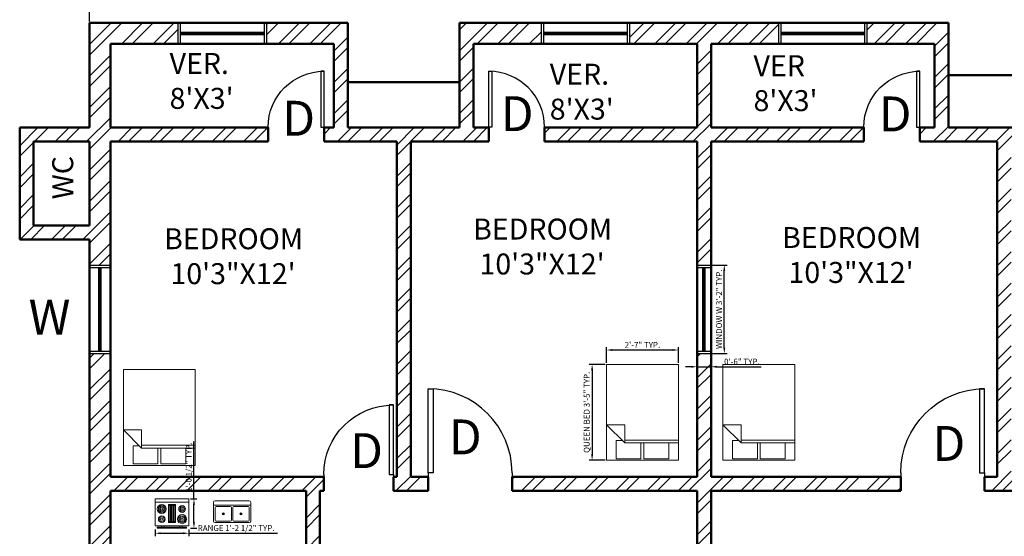
# Model space of a CAD drawing. Units: inches. Extents: x -31485 to -28799, y 18003 to 19130.
# Tile 13 of 15: x -29694 to -29271, y 18604 to 18825. Entities that reach past the tile are written whole.
import ezdxf

# ---------------------------------------------------------------- set-up
doc = ezdxf.new("R2010")
doc.units = ezdxf.units.IN
for name, color, linetype, lineweight in [('A-ANNO-DIMS', 2, 'Continuous', 18), ('A-ANNO-TEXT', 7, 'Continuous', 18), ('A-AREA-IDEN', 7, 'Continuous', 18), ('A-DOOR', 3, 'Continuous', 25), ('A-FLOR-FIXT', 9, 'Continuous', 18), ('A-FURN', 8, 'Continuous', 18), ('A-GLAZ', 4, 'Continuous', 25), ('A-WALL', 7, 'Continuous', 50), ('A-WALL-PATT', 8, 'Continuous', 13)]:
    doc.layers.add(name, color=color, linetype=linetype, lineweight=lineweight)
doc.styles.get("Standard").update_dxf_attribs({"font": 'arial.ttf'})
doc.dimstyles.new('ISO-25', dxfattribs={"dimtxt": 2.5, "dimasz": 2.5, "dimexe": 1.25, "dimexo": 0.625, "dimtad": 1, "dimdec": 0, "dimlunit": 3, "dimtxsty": 'Standard', "dimcen": 2.5, "dimadec": 0, "dimazin": 0, "dimtfac": 1, "dimtdec": 0, "dimtmove": 0, "dimatfit": 3, "dimfxl": 1, "dimarcsym": 0})

# ---------------------------------------------------------------- blocks, each defined once
blk = doc.blocks.new('*U8')
for p, q in [((0, 0), (0, -100)), ((750, 0), (750, -100))]:
    blk.add_line(p, q)
blk.add_lwpolyline([(0, 0), (0, 750), (43.75, 750), (43.75, 0)], close=True)
blk.add_arc((0, 0), 750, 0, 90)
blk = doc.blocks.new('Bed - Queen')
for p, q in [((0, -80.00003), (0, 0)), ((0, 0), (59.99999, 0)), ((59.99999, 0), (59.99999, -80.00003)), ((7.99999, -1.2), (28.79998, -1.2)), ((7.99999, -14.4), (7.99999, -1.2)), ((28.79998, -1.2), (28.79998, -14.4)), ((31.19999, -1.2), (51.99999, -1.2)), ((31.19999, -14.4), (31.19999, -1.2)), ((51.99999, -1.2), (51.99999, -16.4)), ((0, -14.4), (44.8, -14.4)), ((59.99999, -29.6), (44.8, -14.4)), ((44.8, -14.4), (44.8, -29.6)), ((51.99999, -16.4), (46.79936, -16.4)), ((44.8, -16.8), (0, -16.8)), ((44.8, -29.6), (59.99999, -29.6)), ((59.99999, -80.00003), (0, -80.00003))]:
    blk.add_line(p, q)
blk = doc.blocks.new('Range-Oven - 30 in top')
for p, q in [((0, -3), (30, -3)), ((12, -6), (18, -6)), ((13, -20), (13, -6)), ((14, -6), (14, -20)), ((15, -20), (15, -6)), ((16, -6), (16, -20)), ((17, -20), (17, -6)), ((6, -24), (6, -25)), ((8, -25), (8, -24)), ((18, -20), (12, -20)), ((22, -25), (22, -24)), ((24, -24), (24, -25))]:
    blk.add_line(p, q)
for points in [[(0, -24), (0, 0), (30, 0), (30, -24)], [(12, -21), (12, -5), (18, -5), (18, -21)], [(2, -26), (2, -25), (28, -25), (28, -26)]]:
    blk.add_lwpolyline(points, close=True)
for centre, radius in [((6, -9), 4), ((6, -9), 3), ((6, -9), 2), ((6, -9), 1), ((24, -9), 3), ((24, -9), 2), ((24, -9), 1), ((6, -18), 3), ((6, -18), 2), ((6, -18), 1), ((24, -18), 4), ((24, -18), 3), ((24, -18), 2), ((24, -18), 1)]:
    blk.add_circle(centre, radius)
blk = doc.blocks.new('Sink-double - 36 in top')
for p, q in [((-18, -4), (18, -4)), ((-0.75, -18.5), (-0.75, -6.5)), ((0.75, -6.5), (0.75, -18.5))]:
    blk.add_line(p, q)
for points in [[(-16.5, 0), (16.5, 0)], [(-18, -19.5), (-18, -1.5)], [(-16.5, -18.5), (-16.5, -6.5)], [(-15.5, -5.5), (-1.75, -5.5)], [(1.75, -5.5), (15.5, -5.5)], [(16.5, -6.5), (16.5, -18.5)], [(18, -1.5), (18, -19.5)], [(16.5, -21), (-16.5, -21)], [(-1.75, -19.5), (-15.5, -19.5)], [(15.5, -19.5), (1.75, -19.5)]]:
    blk.add_lwpolyline(points)
for centre, radius in [((-8.5, -12.5), 1), ((-8.5, -12.5), 0.5), ((8.5, -12.5), 1), ((8.5, -12.5), 0.5)]:
    blk.add_circle(centre, radius)
for centre, radius, start, end in [((-16.5, -1.5), 1.5, 90, 180), ((16.5, -1.5), 1.5, 0, 90), ((-15.5, -6.5), 1, 90, 180), ((-1.75, -6.5), 1, 0, 90), ((1.75, -6.5), 1, 90, 180), ((15.5, -6.5), 1, 0, 90), ((-15.5, -18.5), 1, 180, 270), ((-1.75, -18.5), 1, 270, 0), ((1.75, -18.5), 1, 180, 270), ((15.5, -18.5), 1, 270, 0), ((-16.5, -19.5), 1.5, 180, 270), ((16.5, -19.5), 1.5, 270, 0)]:
    blk.add_arc(centre, radius, start, end)
blk = doc.blocks.new('*D204')
at = {"layer": 'A-ANNO-DIMS', "color": 0, "lineweight": -2, "transparency": 16777216}
for p, q in [((-29663.82, 18824.74), (-29663.82, 18894.35)), ((-29661.32, 18893.1), (-29118.32, 18893.1)), ((-29115.82, 18824.74), (-29115.82, 18894.35))]:
    blk.add_line(p, q, dxfattribs=at)
at = {"layer": 'A-ANNO-DIMS', "color": 0, "transparency": 16777216}
for points in [[(-29661.32, 18893.52), (-29661.32, 18892.68), (-29663.82, 18893.1)], [(-29118.32, 18893.52), (-29118.32, 18892.68), (-29115.82, 18893.1)]]:
    blk.add_solid(points, dxfattribs=at)
at = {"layer": 'Defpoints', "color": 0, "transparency": 16777216}
for p in [(-29115.82, 18893.1), (-29663.82, 18824.12), (-29115.82, 18824.12)]:
    blk.add_point(p, dxfattribs=at)
at = {"layer": 'A-ANNO-DIMS', "color": 0, "transparency": 16777216, "insert": (-29389.82, 18901.9), "char_height": 2.5, "attachment_point": 5}
blk.add_mtext('{\\H6.4x;45\'-8"}', dxfattribs=at)
blk = doc.blocks.new('WIN-900-W9')
for p, q in [((-29982.21, 18824.12), (-29982.21, 18815.12)), ((-29981.21, 18824.12), (-29981.21, 18815.12)), ((-29945.21, 18824.12), (-29945.21, 18815.12)), ((-29944.21, 18824.12), (-29944.21, 18815.12)), ((-29981.21, 18820.12), (-29945.21, 18820.12)), ((-29981.21, 18819.62), (-29945.21, 18819.62)), ((-29981.21, 18819.12), (-29945.21, 18819.12))]:
    blk.add_line(p, q)
blk = doc.blocks.new('WIN-900-W6')
for p, q in [((-30183.21, 18720.12), (-30177.21, 18720.12)), ((-30183.21, 18719.12), (-30177.21, 18719.12)), ((-30180.71, 18683.12), (-30180.71, 18719.12)), ((-30180.21, 18683.12), (-30180.21, 18719.12)), ((-30179.71, 18683.12), (-30179.71, 18719.12)), ((-30183.21, 18683.12), (-30177.21, 18683.12)), ((-30183.21, 18682.12), (-30177.21, 18682.12))]:
    blk.add_line(p, q)
blk = doc.blocks.new('*D212')
at = {"layer": 'A-ANNO-DIMS', "color": 0, "lineweight": -2, "transparency": 16777216}
for p, q in [((-29396.2, 18720.12), (-29389.87, 18720.12)), ((-29391.12, 18684.62), (-29391.12, 18717.62)), ((-29396.2, 18682.12), (-29389.87, 18682.12))]:
    blk.add_line(p, q, dxfattribs=at)
at = {"layer": 'A-ANNO-DIMS', "color": 0, "transparency": 16777216}
for points in [[(-29391.54, 18717.62), (-29390.7, 18717.62), (-29391.12, 18720.12)], [(-29391.54, 18684.62), (-29390.7, 18684.62), (-29391.12, 18682.12)]]:
    blk.add_solid(points, dxfattribs=at)
at = {"layer": 'Defpoints', "color": 0, "transparency": 16777216}
for p in [(-29396.82, 18720.12), (-29391.12, 18720.12), (-29396.82, 18682.12)]:
    blk.add_point(p, dxfattribs=at)
at = {"layer": 'A-ANNO-DIMS', "color": 0, "transparency": 16777216, "insert": (-29393.04, 18701.12), "char_height": 2.5, "attachment_point": 5, "rotation": 90}
blk.add_mtext('WINDOW W 3\'-2" TYP.', dxfattribs=at)
blk = doc.blocks.new('*D213')
at = {"layer": 'A-ANNO-DIMS', "color": 0, "lineweight": -2, "transparency": 16777216}
for p, q in [((-29402.82, 18681.49), (-29402.82, 18675.17)), ((-29396.82, 18681.49), (-29396.82, 18675.17)), ((-29405.32, 18676.42), (-29407.82, 18676.42)), ((-29402.82, 18676.42), (-29396.82, 18676.42)), ((-29394.32, 18676.42), (-29375.33, 18676.42))]:
    blk.add_line(p, q, dxfattribs=at)
at = {"layer": 'A-ANNO-DIMS', "color": 0, "transparency": 16777216}
for points in [[(-29405.32, 18676.83), (-29405.32, 18676), (-29402.82, 18676.42)], [(-29394.32, 18676.83), (-29394.32, 18676), (-29396.82, 18676.42)]]:
    blk.add_solid(points, dxfattribs=at)
at = {"layer": 'Defpoints', "color": 0, "transparency": 16777216}
for p in [(-29402.82, 18682.12), (-29396.82, 18682.12), (-29396.82, 18676.42)]:
    blk.add_point(p, dxfattribs=at)
at = {"layer": 'A-ANNO-DIMS', "color": 0, "transparency": 16777216, "insert": (-29383.58, 18678.32), "char_height": 2.5, "attachment_point": 5}
blk.add_mtext('0\'-6" TYP.', dxfattribs=at)
blk = doc.blocks.new('*D222')
at = {"layer": 'A-ANNO-DIMS', "color": 0, "lineweight": -2, "transparency": 16777216}
for p, q in [((-29442.35, 18677.44), (-29449.15, 18677.44)), ((-29447.9, 18674.94), (-29447.9, 18638.78)), ((-29442.35, 18636.28), (-29449.15, 18636.28))]:
    blk.add_line(p, q, dxfattribs=at)
at = {"layer": 'A-ANNO-DIMS', "color": 0, "transparency": 16777216}
for points in [[(-29448.32, 18674.94), (-29447.48, 18674.94), (-29447.9, 18677.44)], [(-29448.32, 18638.78), (-29447.48, 18638.78), (-29447.9, 18636.28)]]:
    blk.add_solid(points, dxfattribs=at)
at = {"layer": 'Defpoints', "color": 0, "transparency": 16777216}
for p in [(-29441.73, 18677.44), (-29447.9, 18636.28), (-29441.73, 18636.28)]:
    blk.add_point(p, dxfattribs=at)
at = {"layer": 'A-ANNO-DIMS', "color": 0, "transparency": 16777216, "insert": (-29449.9, 18656.86), "char_height": 2.5, "attachment_point": 5, "rotation": 90}
blk.add_mtext('QUEEN BED 3\'-5" TYP.', dxfattribs=at)
blk = doc.blocks.new('*D223')
at = {"layer": 'A-ANNO-DIMS', "color": 0, "lineweight": -2, "transparency": 16777216}
for p, q in [((-29441.73, 18678.06), (-29441.73, 18684.86)), ((-29410.86, 18678.06), (-29410.86, 18684.86)), ((-29413.36, 18683.61), (-29439.23, 18683.61))]:
    blk.add_line(p, q, dxfattribs=at)
at = {"layer": 'A-ANNO-DIMS', "color": 0, "transparency": 16777216}
for points in [[(-29439.23, 18684.03), (-29439.23, 18683.19), (-29441.73, 18683.61)], [(-29413.36, 18684.03), (-29413.36, 18683.19), (-29410.86, 18683.61)]]:
    blk.add_solid(points, dxfattribs=at)
at = {"layer": 'Defpoints', "color": 0, "transparency": 16777216}
for p in [(-29441.73, 18683.61), (-29441.73, 18677.44), (-29410.86, 18677.44)]:
    blk.add_point(p, dxfattribs=at)
at = {"layer": 'A-ANNO-DIMS', "color": 0, "transparency": 16777216, "insert": (-29426.29, 18685.49), "char_height": 2.5, "attachment_point": 5}
blk.add_mtext('2\'-7" TYP.', dxfattribs=at)
blk = doc.blocks.new('*D250')
at = {"layer": 'A-ANNO-DIMS', "color": 0, "lineweight": -2, "transparency": 16777216}
for p, q in [((-29635.69, 18606.46), (-29635.69, 18603.66)), ((-29633.19, 18604.91), (-29623.64, 18604.91)), ((-29621.14, 18606.46), (-29621.14, 18603.66)), ((-29621.14, 18604.91), (-29583.06, 18604.91))]:
    blk.add_line(p, q, dxfattribs=at)
at = {"layer": 'A-ANNO-DIMS', "color": 0, "transparency": 16777216}
for points in [[(-29633.19, 18605.32), (-29633.19, 18604.49), (-29635.69, 18604.91)], [(-29623.64, 18605.32), (-29623.64, 18604.49), (-29621.14, 18604.91)]]:
    blk.add_solid(points, dxfattribs=at)
at = {"layer": 'Defpoints', "color": 0, "transparency": 16777216}
for p in [(-29635.69, 18607.09), (-29621.14, 18607.09), (-29621.14, 18604.91)]:
    blk.add_point(p, dxfattribs=at)
at = {"layer": 'A-ANNO-DIMS', "color": 0, "transparency": 16777216, "insert": (-29600.85, 18606.82), "char_height": 2.5, "attachment_point": 5}
blk.add_mtext('RANGE 1\'-2 1/2" TYP.', dxfattribs=at)
blk = doc.blocks.new('*D251')
at = {"layer": 'A-ANNO-DIMS', "color": 0, "lineweight": -2, "transparency": 16777216}
for p, q in [((-29618.95, 18619.7), (-29618.95, 18644.28)), ((-29620.51, 18619.7), (-29617.7, 18619.7)), ((-29618.95, 18609.59), (-29618.95, 18617.2)), ((-29620.51, 18607.09), (-29617.7, 18607.09))]:
    blk.add_line(p, q, dxfattribs=at)
at = {"layer": 'A-ANNO-DIMS', "color": 0, "transparency": 16777216}
for points in [[(-29619.37, 18617.2), (-29618.54, 18617.2), (-29618.95, 18619.7)], [(-29619.37, 18609.59), (-29618.54, 18609.59), (-29618.95, 18607.09)]]:
    blk.add_solid(points, dxfattribs=at)
at = {"layer": 'Defpoints', "color": 0, "transparency": 16777216}
for p in [(-29621.14, 18619.7), (-29618.95, 18619.7), (-29621.14, 18607.09)]:
    blk.add_point(p, dxfattribs=at)
at = {"layer": 'A-ANNO-DIMS', "color": 0, "transparency": 16777216, "insert": (-29620.87, 18633.24), "char_height": 2.5, "attachment_point": 5, "rotation": 90}
blk.add_mtext('1\'-0 1/2" TYP.', dxfattribs=at)

msp = doc.modelspace()

# ---------------------------------------------------------------- hatches: boundary and pattern name
at = {"layer": 'A-WALL-PATT'}
h = msp.add_hatch(dxfattribs=at)
h.set_pattern_fill('ANSI32', color=256)
h.set_pattern_definition([(45, (-227.67, 0), (-6.735192, 6.735192), []), (45, (-223.18, 0), (-6.735192, 6.735192), [])])
h.paths.add_polyline_path([(-29507.82, 18213.12), (-29493.82, 18213.12), (-29493.82, 18219.12), (-29507.82, 18219.12), (-29507.82, 18309.12), (-29504.3, 18309.12), (-29504.3, 18315.12), (-29513.82, 18315.12), (-29513.82, 18243.12), (-29654.82, 18243.12), (-29654.82, 18265.36), (-29663.82, 18265.36), (-29663.82, 18180.12), (-29603.32, 18180.12), (-29603.32, 18189.12), (-29654.82, 18189.12), (-29654.82, 18237.12), (-29513.82, 18237.12), (-29513.82, 18189.12), (-29565.32, 18189.12), (-29565.32, 18180.12), (-29507.82, 18180.12)])
h.paths.add_polyline_path([(-29408.82, 18189.12), (-29447.82, 18189.12), (-29447.82, 18371.74), (-29453.82, 18371.74), (-29453.82, 18365.12), (-29476.66, 18365.12), (-29476.66, 18359.12), (-29453.82, 18359.12), (-29453.82, 18315.12), (-29480.3, 18315.12), (-29480.3, 18309.12), (-29453.82, 18309.12), (-29453.82, 18219.12), (-29467.82, 18219.12), (-29467.82, 18213.12), (-29453.82, 18213.12), (-29453.82, 18180.12), (-29408.82, 18180.12)])
h.paths.add_polyline_path([(-29325.82, 18213.12), (-29311.82, 18213.12), (-29311.82, 18219.12), (-29325.82, 18219.12), (-29325.82, 18309.12), (-29298.35, 18309.12), (-29298.35, 18315.12), (-29325.82, 18315.12), (-29325.82, 18359.12), (-29304.41, 18359.12), (-29304.41, 18365.12), (-29325.82, 18365.12), (-29325.82, 18371.25), (-29331.82, 18371.25), (-29331.82, 18189.12), (-29370.82, 18189.12), (-29370.82, 18180.12), (-29325.82, 18180.12)])
h.paths.add_polyline_path([(-29265.82, 18237.12), (-29124.82, 18237.12), (-29124.82, 18189.12), (-29176.32, 18189.12), (-29176.32, 18180.12), (-29115.82, 18180.12), (-29115.82, 18268.84), (-29124.82, 18268.84), (-29124.82, 18243.12), (-29265.82, 18243.12), (-29265.82, 18315.12), (-29274.35, 18315.12), (-29274.35, 18309.12), (-29271.82, 18309.12), (-29271.82, 18219.12), (-29285.82, 18219.12), (-29285.82, 18213.12), (-29271.82, 18213.12), (-29271.82, 18180.12), (-29214.32, 18180.12), (-29214.32, 18189.12), (-29265.82, 18189.12)])
h.paths.add_polyline_path([(-29209.82, 18365.12), (-29262.82, 18365.12), (-29268.41, 18365.12), (-29268.41, 18359.12), (-29209.82, 18359.12)])
h.paths.add_polyline_path([(-29085.82, 18365.12), (-29115.82, 18365.12), (-29115.82, 18400.12), (-29124.82, 18400.12), (-29124.82, 18365.12), (-29171.82, 18365.12), (-29171.82, 18359.12), (-29124.82, 18359.12), (-29124.82, 18306.84), (-29115.82, 18306.84), (-29115.82, 18317.12), (-29085.82, 18317.12)])
h.paths.add_polyline_path([(-29115.82, 18359.12), (-29091.82, 18359.12), (-29091.82, 18323.12), (-29115.82, 18323.12)], flags=16)
h.paths.add_polyline_path([(-29607.82, 18365.12), (-29654.82, 18365.12), (-29654.82, 18400.12), (-29663.82, 18400.12), (-29663.82, 18365.12), (-29693.82, 18365.12), (-29693.82, 18317.12), (-29663.82, 18317.12), (-29663.82, 18303.36), (-29654.82, 18303.36), (-29654.82, 18359.12), (-29607.82, 18359.12)])
h.paths.add_polyline_path([(-29663.82, 18359.12), (-29663.82, 18323.12), (-29687.82, 18323.12), (-29687.82, 18359.12)], flags=16)
h.paths.add_polyline_path([(-29512.66, 18365.12), (-29516.82, 18365.12), (-29569.82, 18365.12), (-29569.82, 18359.12), (-29512.66, 18359.12)])
h.paths.add_polyline_path([(-29654.82, 18473.12), (-29553.73, 18473.12), (-29553.73, 18479.12), (-29564.82, 18479.12), (-29564.82, 18500.25), (-29569.57, 18500.25, -0.011537), (-29570.67, 18500.25), (-29570.82, 18500.25), (-29570.82, 18479.12), (-29675.82, 18479.12), (-29675.82, 18493.12), (-29681.82, 18493.12), (-29681.82, 18473.12), (-29663.82, 18473.12), (-29663.82, 18438.12), (-29654.82, 18438.12)])
h.paths.add_polyline_path([(-29564.82, 18547.44), (-29570.82, 18547.44), (-29570.82, 18539.12), (-29654.82, 18539.12), (-29654.82, 18562.12), (-29663.82, 18562.12), (-29663.82, 18539.12), (-29681.82, 18539.12), (-29681.82, 18519.12), (-29675.82, 18519.12), (-29675.82, 18533.12), (-29570.82, 18533.12), (-29570.82, 18524.25), (-29564.82, 18524.25)])
h.paths.add_polyline_path([(-29563.19, 18629.12), (-29654.82, 18629.12), (-29654.82, 18682.12), (-29663.82, 18682.12), (-29663.82, 18600.12), (-29654.82, 18600.12), (-29654.82, 18623.12), (-29570.82, 18623.12), (-29570.82, 18583.44), (-29566.85, 18583.44), (-29564.82, 18583.44), (-29564.82, 18623.12), (-29563.19, 18623.12)])
h.paths.add_polyline_path([(-29315.33, 18629.12), (-29396.82, 18629.12), (-29396.82, 18682.12), (-29402.82, 18682.12), (-29402.82, 18629.12), (-29482.28, 18629.12), (-29482.28, 18626.12), (-29482.28, 18623.12), (-29402.82, 18623.12), (-29402.82, 18416.12), (-29453.82, 18416.12), (-29453.82, 18407.74), (-29447.82, 18407.74), (-29447.82, 18410.12), (-29331.82, 18410.12), (-29331.82, 18407.25), (-29325.82, 18407.25), (-29325.82, 18416.12), (-29396.82, 18416.12), (-29396.82, 18623.12), (-29315.33, 18623.12)])
h.paths.add_polyline_path([(-29525.82, 18773.12), (-29492.32, 18773.12), (-29492.32, 18779.12), (-29498.82, 18779.12), (-29498.82, 18815.12), (-29469.82, 18815.12), (-29469.82, 18824.12), (-29504.82, 18824.12), (-29504.82, 18779.12), (-29552.82, 18779.12), (-29552.82, 18824.12), (-29587.82, 18824.12), (-29587.82, 18815.12), (-29558.82, 18815.12), (-29558.82, 18779.12), (-29563.08, 18779.12), (-29563.08, 18776.12), (-29563.08, 18773.12), (-29531.82, 18773.12), (-29531.82, 18629.12), (-29533.3, 18629.12), (-29533.3, 18626.12), (-29533.3, 18623.12), (-29518.28, 18623.12), (-29518.28, 18629.12), (-29525.82, 18629.12)])
h.paths.add_polyline_path([(-29654.82, 18779.12), (-29654.82, 18815.12), (-29625.82, 18815.12), (-29625.82, 18824.12), (-29663.82, 18824.12), (-29663.82, 18779.12), (-29693.82, 18779.12), (-29693.82, 18731.12), (-29663.82, 18731.12), (-29663.82, 18720.12), (-29654.82, 18720.12), (-29654.82, 18773.12), (-29587.08, 18773.12), (-29587.08, 18779.12)])
h.paths.add_polyline_path([(-29663.82, 18773.12), (-29663.82, 18737.12), (-29687.82, 18737.12), (-29687.82, 18773.12)], flags=16)
h.paths.add_polyline_path([(-29396.82, 18815.12), (-29367.82, 18815.12), (-29367.82, 18824.12), (-29431.82, 18824.12), (-29431.82, 18815.12), (-29402.82, 18815.12), (-29402.82, 18779.12), (-29468.32, 18779.12), (-29468.32, 18776.12), (-29468.32, 18773.12), (-29402.82, 18773.12), (-29402.82, 18720.12), (-29396.82, 18720.12), (-29396.82, 18773.12), (-29331.17, 18773.12), (-29331.17, 18779.12), (-29396.82, 18779.12)])
h.paths.add_polyline_path([(-29232.68, 18779.12), (-29240.82, 18779.12), (-29240.82, 18815.12), (-29201.82, 18815.12), (-29201.82, 18824.12), (-29246.82, 18824.12), (-29246.82, 18779.12), (-29294.82, 18779.12), (-29294.82, 18824.12), (-29329.82, 18824.12), (-29329.82, 18815.12), (-29300.82, 18815.12), (-29300.82, 18779.12), (-29307.17, 18779.12), (-29307.17, 18776.12), (-29307.17, 18773.12), (-29273.82, 18773.12), (-29273.82, 18629.12), (-29279.33, 18629.12), (-29279.33, 18626.12), (-29279.33, 18623.12), (-29262.04, 18623.12), (-29262.04, 18629.12), (-29267.82, 18629.12), (-29267.82, 18773.12), (-29232.68, 18773.12)])
h.paths.add_polyline_path([(-29085.82, 18779.12), (-29115.82, 18779.12), (-29115.82, 18824.12), (-29163.82, 18824.12), (-29163.82, 18815.12), (-29124.82, 18815.12), (-29124.82, 18779.12), (-29208.68, 18779.12), (-29208.68, 18776.12), (-29208.68, 18773.12), (-29124.82, 18773.12), (-29124.82, 18720.12), (-29115.82, 18720.12), (-29115.82, 18731.12), (-29085.82, 18731.12)])
h.paths.add_polyline_path([(-29115.82, 18773.12), (-29091.82, 18773.12), (-29091.82, 18737.12), (-29115.82, 18737.12)], flags=16)
h.paths.add_polyline_path([(-29115.82, 18682.12), (-29124.82, 18682.12), (-29124.82, 18629.12), (-29226.04, 18629.12), (-29226.04, 18626.12), (-29226.04, 18623.12), (-29214.82, 18623.12), (-29214.82, 18589.35), (-29208.82, 18589.35), (-29208.82, 18623.12), (-29124.82, 18623.12), (-29124.82, 18600.12), (-29115.82, 18600.12)])
h.paths.add_polyline_path([(-29115.82, 18562.12), (-29124.82, 18562.12), (-29124.82, 18539.12), (-29208.82, 18539.12), (-29208.82, 18553.35), (-29211.82, 18553.35), (-29214.82, 18553.35), (-29214.82, 18522.99), (-29208.82, 18522.99), (-29208.82, 18533.12), (-29103.82, 18533.12), (-29103.82, 18519.12), (-29097.82, 18519.12), (-29097.82, 18539.12), (-29115.82, 18539.12)])
h.paths.add_polyline_path([(-29115.82, 18473.12), (-29097.82, 18473.12), (-29097.82, 18493.12), (-29103.82, 18493.12), (-29103.82, 18479.12), (-29208.82, 18479.12), (-29208.82, 18498.99), (-29214.82, 18498.99), (-29214.82, 18479.12), (-29238.82, 18479.12), (-29238.82, 18473.12), (-29124.82, 18473.12), (-29124.82, 18438.12), (-29115.82, 18438.12)])
h.paths.add_polyline_path([(-29513.85, 18245.24), (-29448.79, 18245.24), (-29448.79, 18278.82), (-29513.85, 18278.82)], flags=9)
h.paths.add_polyline_path([(-29331.85, 18241.25), (-29266.79, 18241.25), (-29266.79, 18274.84), (-29331.85, 18274.84)], flags=9)
h.paths.add_polyline_path([(-29095.1, 18330.99), (-29095.1, 18356.44), (-29113.65, 18356.44), (-29113.65, 18330.99)], flags=8)
h.paths.add_polyline_path([(-29666.32, 18333.81), (-29666.32, 18359.25), (-29684.87, 18359.25), (-29684.87, 18333.81)], flags=24)
h.paths.add_polyline_path([(-29665.76, 18745.92), (-29665.76, 18771.37), (-29684.31, 18771.37), (-29684.31, 18745.92)], flags=8)
h.paths.add_polyline_path([(-29093.62, 18744.62), (-29093.62, 18770.06), (-29112.17, 18770.06), (-29112.17, 18744.62)], flags=8)

# ---------------------------------------------------------------- linework, layer by layer
at = {"layer": 'A-WALL'}
for p, q in [((-29663.82, 18824.12), (-29552.82, 18824.12)), ((-29663.82, 18779.12), (-29663.82, 18824.12)), ((-29552.82, 18779.12), (-29552.82, 18824.12)), ((-29504.82, 18779.12), (-29504.82, 18824.12)), ((-29504.82, 18824.12), (-29294.82, 18824.12)), ((-29294.82, 18779.12), (-29294.82, 18824.12)), ((-29654.82, 18815.12), (-29558.82, 18815.12)), ((-29654.82, 18779.12), (-29654.82, 18815.12)), ((-29558.82, 18779.12), (-29558.82, 18815.12)), ((-29498.82, 18779.12), (-29498.82, 18815.12)), ((-29498.82, 18815.12), (-29402.82, 18815.12)), ((-29402.82, 18779.12), (-29402.82, 18815.12)), ((-29396.82, 18779.12), (-29396.82, 18815.12)), ((-29396.82, 18815.12), (-29300.82, 18815.12)), ((-29300.82, 18779.12), (-29300.82, 18815.12)), ((-29552.82, 18798.62), (-29504.82, 18798.62)), ((-29294.82, 18801.62), (-29246.82, 18801.62)), ((-29693.82, 18779.12), (-29663.82, 18779.12)), ((-29693.82, 18731.12), (-29693.82, 18779.12)), ((-29654.82, 18779.12), (-29587.08, 18779.12)), ((-29587.08, 18779.12), (-29587.08, 18773.12)), ((-29563.08, 18779.12), (-29563.08, 18773.12)), ((-29563.08, 18779.12), (-29558.82, 18779.12)), ((-29552.82, 18779.12), (-29504.82, 18779.12)), ((-29498.82, 18779.12), (-29492.32, 18779.12)), ((-29492.32, 18779.12), (-29492.32, 18773.12)), ((-29468.32, 18779.12), (-29468.32, 18773.12)), ((-29468.32, 18779.12), (-29402.82, 18779.12)), ((-29396.82, 18779.12), (-29331.17, 18779.12)), ((-29331.17, 18779.12), (-29331.17, 18773.12)), ((-29307.17, 18779.12), (-29307.17, 18773.12)), ((-29307.17, 18779.12), (-29300.82, 18779.12)), ((-29294.82, 18779.12), (-29246.82, 18779.12)), ((-29687.82, 18773.12), (-29663.82, 18773.12)), ((-29687.82, 18737.12), (-29687.82, 18773.12)), ((-29663.82, 18737.12), (-29663.82, 18773.12)), ((-29654.82, 18629.12), (-29654.82, 18773.12)), ((-29654.82, 18773.12), (-29587.08, 18773.12)), ((-29563.08, 18773.12), (-29531.82, 18773.12)), ((-29531.82, 18629.12), (-29531.82, 18773.12)), ((-29525.82, 18629.12), (-29525.82, 18773.12)), ((-29525.82, 18773.12), (-29492.32, 18773.12)), ((-29468.32, 18773.12), (-29402.82, 18773.12)), ((-29402.82, 18629.12), (-29402.82, 18773.12)), ((-29396.82, 18629.12), (-29396.82, 18773.12)), ((-29396.82, 18773.12), (-29331.17, 18773.12)), ((-29307.17, 18773.12), (-29273.82, 18773.12)), ((-29273.82, 18629.12), (-29273.82, 18773.12)), ((-29687.82, 18737.12), (-29663.82, 18737.12)), ((-29693.82, 18731.12), (-29663.82, 18731.12)), ((-29663.82, 18539.12), (-29663.82, 18731.12)), ((-29654.82, 18629.12), (-29563.19, 18629.12)), ((-29563.19, 18623.12), (-29563.19, 18629.12)), ((-29533.3, 18629.12), (-29533.3, 18623.12)), ((-29533.3, 18629.12), (-29531.82, 18629.12)), ((-29525.82, 18629.12), (-29518.28, 18629.12)), ((-29518.28, 18629.12), (-29518.28, 18623.12)), ((-29482.28, 18629.12), (-29482.28, 18623.12)), ((-29482.28, 18629.12), (-29402.82, 18629.12)), ((-29396.82, 18629.12), (-29315.33, 18629.12)), ((-29315.33, 18629.12), (-29315.33, 18623.12)), ((-29279.33, 18629.12), (-29279.33, 18623.12)), ((-29279.33, 18629.12), (-29273.82, 18629.12)), ((-29654.82, 18623.12), (-29570.82, 18623.12)), ((-29654.82, 18539.12), (-29654.82, 18623.12)), ((-29570.82, 18583.44), (-29570.82, 18623.12)), ((-29564.82, 18623.12), (-29563.19, 18623.12)), ((-29564.82, 18583.44), (-29564.82, 18623.12)), ((-29533.3, 18623.12), (-29518.28, 18623.12)), ((-29482.28, 18623.12), (-29402.82, 18623.12)), ((-29402.82, 18416.12), (-29402.82, 18623.12)), ((-29396.82, 18416.12), (-29396.82, 18623.12)), ((-29396.82, 18623.12), (-29315.33, 18623.12)), ((-29279.33, 18623.12), (-29262.04, 18623.12))]:
    msp.add_line(p, q, dxfattribs=at)

# ---------------------------------------------------------------- block references
at = {"layer": 'A-DOOR'}
for p, xscale, yscale, zscale in [((-29563.08, 18779.32), -0.0320000014788075, 0.0320000014788075, 0.0320000014788075), ((-29492.32, 18779.32), 0.0320000000000009, 0.0320000000000009, 0.0320000000000009), ((-29307.17, 18779.32), -0.0320000014788075, 0.0320000014788075, 0.0320000014788075), ((-29518.28, 18630.92), 0.0480000000000013, 0.0480000000000013, 0.0480000000000013), ((-29279.33, 18630.92), -0.0479999987086216, 0.0479999987086216, 0.0479999987086216), ((-29533.3, 18630.1), -0.0398603435773381, 0.0398603435773381, 0.0398603435773381)]:
    msp.add_blockref('*U8', p, dxfattribs=dict(at, xscale=xscale, yscale=yscale, zscale=zscale))
at = {"layer": 'A-FLOR-FIXT'}
for name, p, xscale, yscale, zscale in [('Range-Oven - 30 in top', (-29635.69, 18619.7), 0.4852446628127246, 0.4852446628127246, 0.4852446628127246), ('Sink-double - 36 in top', (-29602.55, 18618.82), 0.4446151646272686, 0.4446151646272686, 0.4446151646272686)]:
    msp.add_blockref(name, p, dxfattribs=dict(at, xscale=xscale, yscale=yscale, zscale=zscale))
at = {"layer": 'A-FURN', "xscale": 0.5144931166195136, "yscale": 0.5144931166195136, "zscale": 0.5144931166195136, "rotation": 180}
for p in [(-29410.86, 18636.28), (-29360.84, 18636.28), (-29618.37, 18634.05)]:
    msp.add_blockref('Bed - Queen', p, dxfattribs=at)
at = {"layer": 'A-GLAZ'}
for name, p in [('WIN-900-W9', (356.38, 0)), ('WIN-900-W9', (512.38, 0)), ('WIN-900-W9', (614.38, 0)), ('WIN-900-W6', (780.38, 0))]:
    msp.add_blockref(name, p, dxfattribs=at)
at = {"layer": 'A-GLAZ', "rotation": 89.9999999999743}
msp.add_blockref('WIN-900-W9', (-10839.7, 48664.32), dxfattribs=at)

# ---------------------------------------------------------------- texts
at = {"layer": 'A-ANNO-TEXT', "char_height": 15, "attachment_point": 1}
for s, insert in [('{D}', (-29581, 18790.64)), ('{D}', (-29487.14, 18792.61)), ('{D}', (-29324.78, 18792.5)), ('{W}', (-29690, 18705.25)), ('{D}', (-29509.43, 18653.78)), ('{D}', (-29301.68, 18650.98)), ('{D}', (-29551.85, 18647.89))]:
    msp.add_mtext_dynamic_manual_height_columns(s, width=1534.0875, gutter_width=12.5, heights=[0], dxfattribs=dict(at, insert=insert))
at = {"layer": 'A-AREA-IDEN', "char_height": 9, "attachment_point": 1}
for s, insert in [("{     VER.\\P     8'X3'}", (-29643.18, 18811.19)), ("{    VER\\P    8'X3'}", (-29389.57, 18810.22)), ("{VER.\\P8'X3'}", (-29466.1, 18806.57)), ('{BEDROOM\\P 10\'3"X12\'}', (-29499.04, 18740.06)), ('{BEDROOM\\P 10\'3"X12\'}', (-29631.8, 18735.9)), ('{BEDROOM\\P 10\'3"X12\'}', (-29366.29, 18736.42))]:
    msp.add_mtext_dynamic_manual_height_columns(s, width=988.498, gutter_width=12.5, heights=[0], dxfattribs=dict(at, insert=insert))
at = {"layer": 'A-AREA-IDEN', "insert": (-29679.83, 18748.32), "char_height": 9, "attachment_point": 1, "rotation": 90}
msp.add_mtext_dynamic_manual_height_columns('{WC}', width=988.498, gutter_width=12.5, heights=[0], dxfattribs=at)

# ---------------------------------------------------------------- dimensions: what is measured, and where the dimension line sits
at = {"layer": 'A-ANNO-DIMS'}
for base, p1, p2, text, override, picture, middle in [((-29115.82, 18893.1), (-29663.82, 18824.12), (-29115.82, 18824.12), '{\\H6.4x;<>}', {"dimclrd": 0, "dimclre": 0, "dimclrt": 0}, '*D204', (-29389.82, 18901.9)), ((-29396.82, 18676.42), (-29402.82, 18682.12), (-29396.82, 18682.12), '<> TYP.', {"dimdec": 1, "dimlfac": 1, "dimrnd": 0, "dimzin": 1, "dimdsep": 46, "dimlunit": 4, "dimfrac": 2}, '*D213', (-29383.58, 18678.32)), ((-29621.1354, 18604.905), (-29635.6927, 18607.0886), (-29621.1354, 18607.0886), 'RANGE <> TYP.', {"dimdec": 1, "dimlfac": 1, "dimrnd": 0, "dimzin": 1, "dimdsep": 46, "dimlunit": 4, "dimfrac": 2}, '*D250', (-29600.8481, 18606.8226))]:
    dim = msp.add_linear_dim(base=base, p1=p1, p2=p2, text=text, dimstyle='ISO-25', override=override, dxfattribs=at)
    dim.commit()
    dim.dimension.update_dxf_attribs({"geometry": picture, "text_midpoint": middle})
for base, p1, p2, angle, text, picture, middle in [((-29391.12, 18720.12), (-29396.82, 18682.12), (-29396.82, 18720.12), 90, 'WINDOW W <> TYP.', '*D212', (-29393.04, 18701.12)), ((-29441.73, 18683.61), (-29410.86, 18677.44), (-29441.73, 18677.44), 180, '<> TYP.', '*D223', (-29426.29, 18685.49)), ((-29447.9, 18636.28), (-29441.73, 18677.44), (-29441.73, 18636.28), 270, 'QUEEN BED <> TYP.', '*D222', (-29449.9, 18656.86)), ((-29618.95, 18619.7), (-29621.14, 18607.09), (-29621.14, 18619.7), 90, '<> TYP.', '*D251', (-29620.87, 18633.24))]:
    dim = msp.add_linear_dim(base=base, p1=p1, p2=p2, angle=angle, text=text, dimstyle='ISO-25', override={"dimdec": 1, "dimlfac": 1, "dimrnd": 0, "dimzin": 1, "dimdsep": 46, "dimlunit": 4, "dimfrac": 2}, dxfattribs=at)
    dim.commit()
    dim.dimension.update_dxf_attribs({"geometry": picture, "text_midpoint": middle})

doc.saveas('drawing.dxf')
